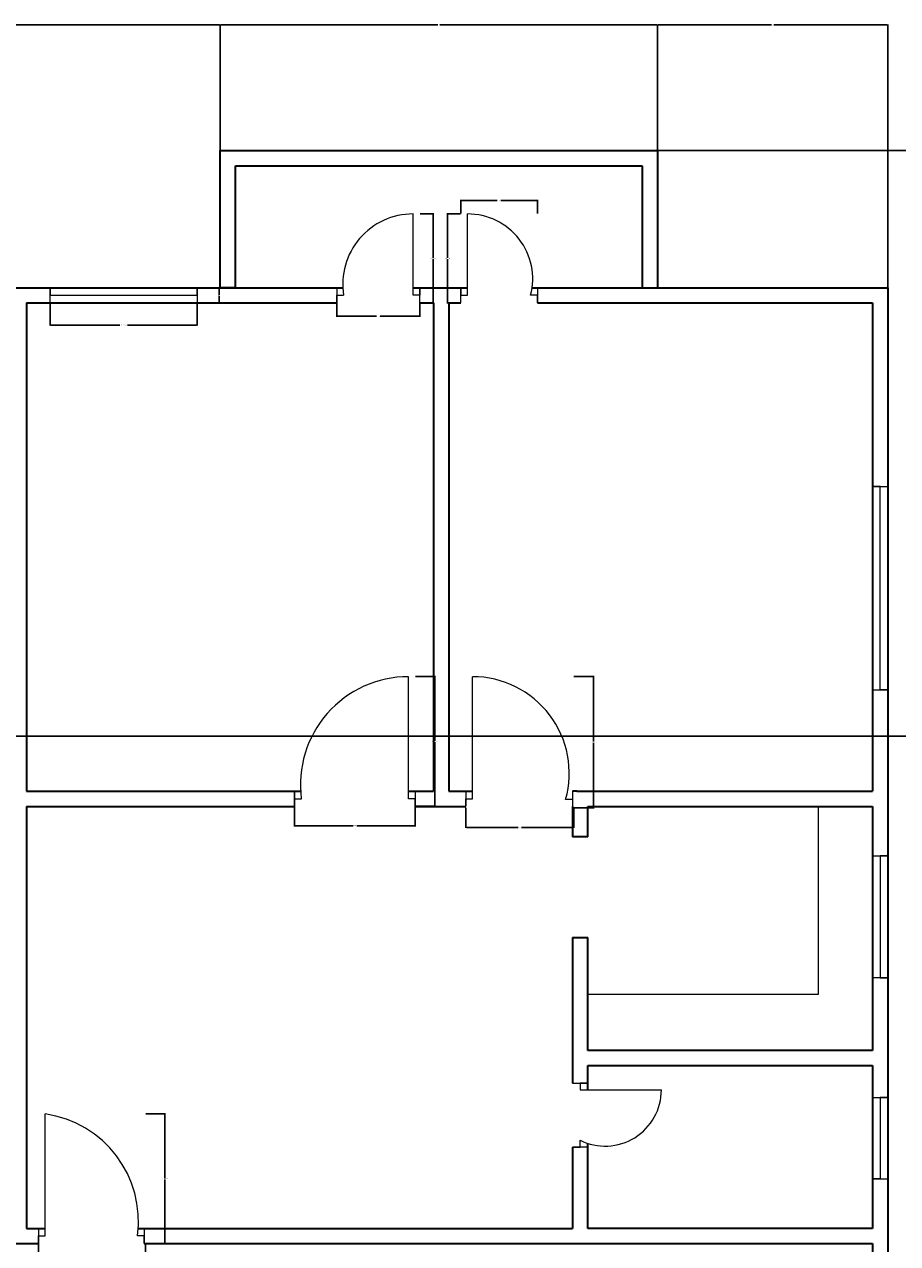
# Model space of a CAD drawing. Units: inches. Extents: x 1944 to 3454, y 1352 to 3055.
# Tile 14 of 17: x 2903 to 3160, y 1900 to 2260. Entities that reach past the tile are written whole.
import ezdxf

# ---------------------------------------------------------------- set-up
doc = ezdxf.new("R2010")
doc.units = ezdxf.units.IN
for name, color, linetype, lineweight in [('A-ANNO-DIMS', 2, 'Continuous', 18), ('A-ANNO-SYMB', 7, 'Continuous', 25), ('A-DOOR', 3, 'Continuous', 20), ('A-FLOR-CASE', 8, 'Continuous', 20), ('A-GLAZ', 4, 'Continuous', 18), ('A-WALL', 7, 'Continuous', 35)]:
    doc.layers.add(name, color=color, linetype=linetype, lineweight=lineweight)
doc.styles.get("Standard").update_dxf_attribs({"font": 'arial.ttf'})
doc.dimstyles.get("Standard").update_dxf_attribs({"dimtxt": 0.18, "dimasz": 0.18, "dimexe": 0.18, "dimexo": 0.0625, "dimgap": 0.09, "dimtad": 0, "dimtih": 1, "dimtoh": 1, "dimdec": 4, "dimzin": 0, "dimdsep": 46, "dimtxsty": 'Standard', "dimcen": 0.09, "dimadec": 0, "dimazin": 0, "dimtfac": 1, "dimtdec": 4, "dimtofl": 0, "dimtmove": 0, "dimatfit": 3, "dimfxl": 1, "dimtolj": 1, "dimtzin": 0, "dimarcsym": 0})

# ---------------------------------------------------------------- blocks, each defined once
blk = doc.blocks.new('DOOR-SWING-36IN-01')
for p, q in [((33.61, 2.25), (33.61, 38.25)), ((0, 4.5), (0, 0)), ((0, 0), (0, 4.5)), ((0, 4.5), (0, 2.25)), ((35.61, 4.5), (35.61, 0)), ((0, 2.25), (2, 2.25)), ((35.61, 2.25), (33.61, 2.25)), ((35.61, 0), (35.61, 2.25))]:
    blk.add_line(p, q)
blk.add_arc((33.61, 6.37), 31.88, 90, 187.4328)
blk = doc.blocks.new('DOOR-SWING-36IN-02')
for p, q in [((2, 2.65), (2, 38.65)), ((0, 4.9), (0, 0.4)), ((31.45, 4.9), (31.45, 0)), ((0, 0.4), (0, 2.65)), ((0, 2.65), (2, 2.65)), ((31.45, 2.45), (29.45, 2.45))]:
    blk.add_line(p, q)
blk.add_arc((2, 10.14), 28.51, 344.3464, 90)
blk = doc.blocks.new('DOOR-SWING-24IN-03')
for p, q in [((22.49, 2.25), (22.49, 26.25)), ((0, 4.5), (0, 0)), ((24.49, 0), (24.49, 4.5)), ((24.49, 4.5), (24.49, 2.25)), ((0, 0), (0, 2.25)), ((0, 2.25), (2, 2.25)), ((24.49, 2.25), (22.49, 2.25))]:
    blk.add_line(p, q)
blk.add_arc((22.49, 5.5), 20.75, 90, 189.0124)
blk = doc.blocks.new('DOOR-SWING-24IN-04')
for p, q in [((2, 2.25), (2, 26.25)), ((0, 0), (0, 4.5)), ((0, 4.5), (0, 2.25)), ((22.61, 4.5), (22.61, 0)), ((0, 2.25), (2, 2.25)), ((22.61, 2.25), (20.61, 2.25)), ((22.61, 0), (22.61, 2.25))]:
    blk.add_line(p, q)
blk.add_arc((2.1, 7.11), 19.14, 345.2922, 90.304)
blk = doc.blocks.new('DOOR-SWING-24IN-05')
for p, q in [((0, 18.87), (4.5, 18.87)), ((4.5, 18.87), (2.25, 18.87)), ((2.25, 18.87), (2.25, 16.87)), ((2.25, 16.87), (26.25, 16.87)), ((4.5, 0), (0, 0)), ((0, 0), (2.25, 0)), ((2.25, 0), (2.25, 2))]:
    blk.add_line(p, q)
blk.add_arc((9.64, 16.87), 16.61, 243.5781, 0)
blk = doc.blocks.new('DOOR-SWING-36IN-09')
for p, q in [((2, 2.25), (2, 38.25)), ((0, 4.5), (0, 0)), ((31.24, 4.5), (31.24, 0)), ((0, 0), (0, 2.25)), ((0, 2.25), (2, 2.25)), ((31.24, 2.25), (29.24, 2.25)), ((31.24, 0), (31.24, 2.25))]:
    blk.add_line(p, q)
blk.add_arc((-2.49, 6.55), 32.02, 352.2825, 81.9468)
blk = doc.blocks.new('WINDOW-PLAN-60.00IN-02')
for p, q in [((2.25, 60), (0, 60)), ((0, 60), (4.5, 60)), ((2.25, 0), (2.25, 60)), ((0, 0), (4.5, 0)), ((4.5, 0), (2.25, 0))]:
    blk.add_line(p, q)
blk = doc.blocks.new('WINDOW-PLAN-24.00IN-01')
for p, q in [((2.25, 24), (0, 24)), ((0, 24), (4.5, 24)), ((2.25, 0), (2.25, 24)), ((0, 0), (4.5, 0)), ((4.5, 0), (2.25, 0))]:
    blk.add_line(p, q)
blk = doc.blocks.new('WINDOW-PLAN-36.00IN-02')
for p, q in [((0, 36), (4.5, 36)), ((4.5, 36), (2.25, 36)), ((2.25, 36), (2.25, 0)), ((4.5, 0), (0, 0)), ((2.25, 0), (4.5, 0))]:
    blk.add_line(p, q)
blk = doc.blocks.new('WINDOW-PLAN-43.38IN-01')
for p, q in [((0, 0), (0, 4.5)), ((0, 4.5), (0, 2.25)), ((43.38, 2.25), (43.38, 4.5)), ((43.38, 4.5), (43.38, 0)), ((0, 2.25), (43.38, 2.25))]:
    blk.add_line(p, q)
blk = doc.blocks.new('*D88')
at = {"layer": 'A-ANNO-DIMS', "color": 0, "lineweight": -2, "transparency": 16777216}
for p, q in [((2910.28, 2177.53), (2910.28, 2170.91)), ((2953.65, 2177.53), (2953.65, 2170.91)), ((2910.46, 2171.09), (2930.85, 2171.09)), ((2953.47, 2171.09), (2933.08, 2171.09))]:
    blk.add_line(p, q, dxfattribs=at)
at = {"layer": 'A-ANNO-DIMS', "color": 0, "transparency": 16777216}
for points in [[(2910.46, 2171.12), (2910.46, 2171.06), (2910.28, 2171.09)], [(2953.47, 2171.12), (2953.47, 2171.06), (2953.65, 2171.09)]]:
    blk.add_solid(points, dxfattribs=at)
at = {"layer": 'Defpoints', "color": 0, "transparency": 16777216}
for p in [(2910.28, 2177.6), (2953.65, 2177.6), (2953.65, 2171.09)]:
    blk.add_point(p, dxfattribs=at)
at = {"layer": 'A-ANNO-DIMS', "color": 0, "transparency": 16777216, "insert": (2931.96, 2171.09), "char_height": 0.18, "attachment_point": 5}
blk.add_mtext('\\A1;WINDOW 43 TYP.', dxfattribs=at)
blk = doc.blocks.new('*D89')
at = {"layer": 'A-ANNO-DIMS', "color": 0, "lineweight": -2, "transparency": 16777216}
for p, q in [((2953.72, 2182.1), (2960.34, 2182.1)), ((2960.16, 2181.92), (2960.16, 2180.03)), ((2960.16, 2177.78), (2960.16, 2179.66)), ((2953.72, 2177.6), (2960.34, 2177.6))]:
    blk.add_line(p, q, dxfattribs=at)
at = {"layer": 'A-ANNO-DIMS', "color": 0, "transparency": 16777216}
for points in [[(2960.13, 2181.92), (2960.19, 2181.92), (2960.16, 2182.1)], [(2960.13, 2177.78), (2960.19, 2177.78), (2960.16, 2177.6)]]:
    blk.add_solid(points, dxfattribs=at)
at = {"layer": 'Defpoints', "color": 0, "transparency": 16777216}
for p in [(2953.65, 2182.1), (2960.16, 2182.1), (2953.65, 2177.6)]:
    blk.add_point(p, dxfattribs=at)
at = {"layer": 'A-ANNO-DIMS', "color": 0, "transparency": 16777216, "insert": (2960.16, 2179.85), "char_height": 0.18, "attachment_point": 5}
blk.add_mtext('\\A1;5 TYP.', dxfattribs=at)
blk = doc.blocks.new('*D92')
at = {"layer": 'A-ANNO-DIMS', "color": 0, "lineweight": -2, "transparency": 16777216}
for p, q in [((3018.08, 2067.35), (3023.94, 2067.35)), ((3023.76, 2067.17), (3023.76, 2048.4)), ((3023.76, 2029.28), (3023.76, 2048.04)), ((3018.08, 2029.1), (3023.94, 2029.1))]:
    blk.add_line(p, q, dxfattribs=at)
at = {"layer": 'A-ANNO-DIMS', "color": 0, "transparency": 16777216}
for points in [[(3023.73, 2067.17), (3023.79, 2067.17), (3023.76, 2067.35)], [(3023.73, 2029.28), (3023.79, 2029.28), (3023.76, 2029.1)]]:
    blk.add_solid(points, dxfattribs=at)
at = {"layer": 'Defpoints', "color": 0, "transparency": 16777216}
for p in [(3018.02, 2067.35), (3023.76, 2067.35), (3018.02, 2029.1)]:
    blk.add_point(p, dxfattribs=at)
at = {"layer": 'A-ANNO-DIMS', "color": 0, "transparency": 16777216, "insert": (3023.76, 2048.22), "char_height": 0.18, "attachment_point": 5}
blk.add_mtext('\\A1;SWING 38 TYP.', dxfattribs=at)
blk = doc.blocks.new('*D93')
at = {"layer": 'A-ANNO-DIMS', "color": 0, "lineweight": -2, "transparency": 16777216}
for p, q in [((2982.41, 2029.03), (2982.41, 2023.18)), ((3018.02, 2029.03), (3018.02, 2023.18)), ((2982.59, 2023.36), (2999.69, 2023.36)), ((3017.84, 2023.36), (3000.74, 2023.36))]:
    blk.add_line(p, q, dxfattribs=at)
at = {"layer": 'A-ANNO-DIMS', "color": 0, "transparency": 16777216}
for points in [[(2982.59, 2023.39), (2982.59, 2023.33), (2982.41, 2023.36)], [(3017.84, 2023.39), (3017.84, 2023.33), (3018.02, 2023.36)]]:
    blk.add_solid(points, dxfattribs=at)
at = {"layer": 'Defpoints', "color": 0, "transparency": 16777216}
for p in [(2982.41, 2029.1), (3018.02, 2029.1), (3018.02, 2023.36)]:
    blk.add_point(p, dxfattribs=at)
at = {"layer": 'A-ANNO-DIMS', "color": 0, "transparency": 16777216, "insert": (3000.21, 2023.36), "char_height": 0.18, "attachment_point": 5}
blk.add_mtext('\\A1;36 TYP.', dxfattribs=at)
blk = doc.blocks.new('*D94')
at = {"layer": 'A-ANNO-DIMS', "color": 0, "lineweight": -2, "transparency": 16777216}
for p, q in [((3064.84, 2067.35), (3070.76, 2067.35)), ((3070.58, 2067.17), (3070.58, 2048.21)), ((3070.58, 2028.88), (3070.58, 2047.84)), ((3064.84, 2028.7), (3070.76, 2028.7))]:
    blk.add_line(p, q, dxfattribs=at)
at = {"layer": 'A-ANNO-DIMS', "color": 0, "transparency": 16777216}
for points in [[(3070.55, 2067.17), (3070.61, 2067.17), (3070.58, 2067.35)], [(3070.55, 2028.88), (3070.61, 2028.88), (3070.58, 2028.7)]]:
    blk.add_solid(points, dxfattribs=at)
at = {"layer": 'Defpoints', "color": 0, "transparency": 16777216}
for p in [(3064.78, 2067.35), (3070.58, 2067.35), (3064.78, 2028.7)]:
    blk.add_point(p, dxfattribs=at)
at = {"layer": 'A-ANNO-DIMS', "color": 0, "transparency": 16777216, "insert": (3070.58, 2048.02), "char_height": 0.18, "attachment_point": 5}
blk.add_mtext('\\A1;SWING 39 TYP.', dxfattribs=at)
blk = doc.blocks.new('*D95')
at = {"layer": 'A-ANNO-DIMS', "color": 0, "lineweight": -2, "transparency": 16777216}
for p, q in [((3032.93, 2028.64), (3032.93, 2022.72)), ((3064.78, 2028.64), (3064.78, 2022.72)), ((3033.11, 2022.9), (3048.33, 2022.9)), ((3064.6, 2022.9), (3049.38, 2022.9))]:
    blk.add_line(p, q, dxfattribs=at)
at = {"layer": 'A-ANNO-DIMS', "color": 0, "transparency": 16777216}
for points in [[(3033.11, 2022.93), (3033.11, 2022.87), (3032.93, 2022.9)], [(3064.6, 2022.93), (3064.6, 2022.87), (3064.78, 2022.9)]]:
    blk.add_solid(points, dxfattribs=at)
at = {"layer": 'Defpoints', "color": 0, "transparency": 16777216}
for p in [(3032.93, 2028.7), (3064.78, 2028.7), (3064.78, 2022.9)]:
    blk.add_point(p, dxfattribs=at)
at = {"layer": 'A-ANNO-DIMS', "color": 0, "transparency": 16777216, "insert": (3048.85, 2022.9), "char_height": 0.18, "attachment_point": 5}
blk.add_mtext('\\A1;32 TYP.', dxfattribs=at)
blk = doc.blocks.new('*D108')
at = {"layer": 'A-ANNO-DIMS', "color": 0, "lineweight": -2, "transparency": 16777216}
for p, q in [((2938.5, 1938.35), (2944.35, 1938.35)), ((2944.17, 1938.17), (2944.17, 1919.4)), ((2944.17, 1900.28), (2944.17, 1919.04)), ((2938.5, 1900.1), (2944.35, 1900.1))]:
    blk.add_line(p, q, dxfattribs=at)
at = {"layer": 'A-ANNO-DIMS', "color": 0, "transparency": 16777216}
for points in [[(2944.14, 1938.17), (2944.2, 1938.17), (2944.17, 1938.35)], [(2944.14, 1900.28), (2944.2, 1900.28), (2944.17, 1900.1)]]:
    blk.add_solid(points, dxfattribs=at)
at = {"layer": 'Defpoints', "color": 0, "transparency": 16777216}
for p in [(2938.44, 1938.35), (2944.17, 1938.35), (2938.44, 1900.1)]:
    blk.add_point(p, dxfattribs=at)
at = {"layer": 'A-ANNO-DIMS', "color": 0, "transparency": 16777216, "insert": (2944.17, 1919.22), "char_height": 0.18, "attachment_point": 5}
blk.add_mtext('\\A1;SWING 38 TYP.', dxfattribs=at)
blk = doc.blocks.new('*D109')
at = {"layer": 'A-ANNO-DIMS', "color": 0, "lineweight": -2, "transparency": 16777216}
for p, q in [((2906.83, 1900.03), (2906.83, 1894.18)), ((2938.44, 1900.03), (2938.44, 1894.18)), ((2907.01, 1894.36), (2922.11, 1894.36)), ((2938.26, 1894.36), (2923.16, 1894.36))]:
    blk.add_line(p, q, dxfattribs=at)
at = {"layer": 'A-ANNO-DIMS', "color": 0, "transparency": 16777216}
for points in [[(2907.01, 1894.39), (2907.01, 1894.33), (2906.83, 1894.36)], [(2938.26, 1894.39), (2938.26, 1894.33), (2938.44, 1894.36)]]:
    blk.add_solid(points, dxfattribs=at)
at = {"layer": 'Defpoints', "color": 0, "transparency": 16777216}
for p in [(2906.83, 1900.1), (2938.44, 1900.1), (2938.44, 1894.36)]:
    blk.add_point(p, dxfattribs=at)
at = {"layer": 'A-ANNO-DIMS', "color": 0, "transparency": 16777216, "insert": (2922.63, 1894.36), "char_height": 0.18, "attachment_point": 5}
blk.add_mtext('\\A1;32 TYP.', dxfattribs=at)
blk = doc.blocks.new('*D120')
at = {"layer": 'A-ANNO-DIMS', "color": 0, "lineweight": -2, "transparency": 16777216}
for p, q in [((3019.44, 2203.85), (3023.5, 2203.85)), ((3023.32, 2203.67), (3023.32, 2190.9)), ((3023.32, 2177.78), (3023.32, 2190.54)), ((3019.44, 2177.6), (3023.5, 2177.6))]:
    blk.add_line(p, q, dxfattribs=at)
at = {"layer": 'A-ANNO-DIMS', "color": 0, "transparency": 16777216}
for points in [[(3023.29, 2203.67), (3023.35, 2203.67), (3023.32, 2203.85)], [(3023.29, 2177.78), (3023.35, 2177.78), (3023.32, 2177.6)]]:
    blk.add_solid(points, dxfattribs=at)
at = {"layer": 'Defpoints', "color": 0, "transparency": 16777216}
for p in [(3019.38, 2203.85), (3023.32, 2203.85), (3019.38, 2177.6)]:
    blk.add_point(p, dxfattribs=at)
at = {"layer": 'A-ANNO-DIMS', "color": 0, "transparency": 16777216, "insert": (3023.32, 2190.72), "char_height": 0.18, "attachment_point": 5}
blk.add_mtext('\\A1;SWING 26 TYP.', dxfattribs=at)
blk = doc.blocks.new('*D121')
at = {"layer": 'A-ANNO-DIMS', "color": 0, "lineweight": -2, "transparency": 16777216}
for p, q in [((2994.89, 2177.53), (2994.89, 2173.48)), ((3019.38, 2177.53), (3019.38, 2173.48)), ((2995.07, 2173.66), (3006.6, 2173.66)), ((3019.2, 2173.66), (3007.66, 2173.66))]:
    blk.add_line(p, q, dxfattribs=at)
at = {"layer": 'A-ANNO-DIMS', "color": 0, "transparency": 16777216}
for points in [[(2995.07, 2173.69), (2995.07, 2173.63), (2994.89, 2173.66)], [(3019.2, 2173.69), (3019.2, 2173.63), (3019.38, 2173.66)]]:
    blk.add_solid(points, dxfattribs=at)
at = {"layer": 'Defpoints', "color": 0, "transparency": 16777216}
for p in [(2994.89, 2177.6), (3019.38, 2177.6), (3019.38, 2173.66)]:
    blk.add_point(p, dxfattribs=at)
at = {"layer": 'A-ANNO-DIMS', "color": 0, "transparency": 16777216, "insert": (3007.13, 2173.66), "char_height": 0.18, "attachment_point": 5}
blk.add_mtext('\\A1;24 TYP.', dxfattribs=at)
blk = doc.blocks.new('*D122')
at = {"layer": 'A-ANNO-DIMS', "color": 0, "lineweight": -2, "transparency": 16777216}
for p, q in [((3031.36, 2203.88), (3027.3, 2203.88)), ((3027.48, 2203.7), (3027.48, 2190.92)), ((3027.48, 2177.78), (3027.48, 2190.55)), ((3031.36, 2177.6), (3027.3, 2177.6))]:
    blk.add_line(p, q, dxfattribs=at)
at = {"layer": 'A-ANNO-DIMS', "color": 0, "transparency": 16777216}
for points in [[(3027.45, 2203.7), (3027.51, 2203.7), (3027.48, 2203.88)], [(3027.45, 2177.78), (3027.51, 2177.78), (3027.48, 2177.6)]]:
    blk.add_solid(points, dxfattribs=at)
at = {"layer": 'Defpoints', "color": 0, "transparency": 16777216}
for p in [(3027.48, 2203.88), (3031.42, 2203.88), (3031.42, 2177.6)]:
    blk.add_point(p, dxfattribs=at)
at = {"layer": 'A-ANNO-DIMS', "color": 0, "transparency": 16777216, "insert": (3027.48, 2190.74), "char_height": 0.18, "attachment_point": 5}
blk.add_mtext('\\A1;SWING 26 TYP.', dxfattribs=at)
blk = doc.blocks.new('*D123')
at = {"layer": 'A-ANNO-DIMS', "color": 0, "lineweight": -2, "transparency": 16777216}
for p, q in [((3031.42, 2203.94), (3031.42, 2208)), ((3031.6, 2207.82), (3042.2, 2207.82)), ((3053.85, 2207.82), (3043.26, 2207.82)), ((3054.03, 2203.94), (3054.03, 2208))]:
    blk.add_line(p, q, dxfattribs=at)
at = {"layer": 'A-ANNO-DIMS', "color": 0, "transparency": 16777216}
for points in [[(3031.6, 2207.85), (3031.6, 2207.79), (3031.42, 2207.82)], [(3053.85, 2207.85), (3053.85, 2207.79), (3054.03, 2207.82)]]:
    blk.add_solid(points, dxfattribs=at)
at = {"layer": 'Defpoints', "color": 0, "transparency": 16777216}
for p in [(3054.03, 2207.82), (3031.42, 2203.88), (3054.03, 2203.88)]:
    blk.add_point(p, dxfattribs=at)
at = {"layer": 'A-ANNO-DIMS', "color": 0, "transparency": 16777216, "insert": (3042.73, 2207.82), "char_height": 0.18, "attachment_point": 5}
blk.add_mtext('\\A1;23 TYP.', dxfattribs=at)
blk = doc.blocks.new('*D187')
at = {"layer": 'A-ANNO-DIMS', "color": 0, "lineweight": -2, "transparency": 16777216}
for p, q in [((3089.53, 2222.6), (3245.46, 2222.6)), ((3245.28, 2222.42), (3245.28, 1856.28)), ((3245.28, 1489.78), (3245.28, 1855.91)), ((3093.18, 1489.6), (3245.46, 1489.6))]:
    blk.add_line(p, q, dxfattribs=at)
at = {"layer": 'A-ANNO-DIMS', "color": 0, "transparency": 16777216}
for points in [[(3245.25, 2222.42), (3245.31, 2222.42), (3245.28, 2222.6)], [(3245.25, 1489.78), (3245.31, 1489.78), (3245.28, 1489.6)]]:
    blk.add_solid(points, dxfattribs=at)
at = {"layer": 'Defpoints', "color": 0, "transparency": 16777216}
for p in [(3089.47, 2222.6), (3245.28, 2222.6), (3093.12, 1489.6)]:
    blk.add_point(p, dxfattribs=at)
at = {"layer": 'A-ANNO-DIMS', "color": 0, "transparency": 16777216, "insert": (3245.28, 1856.1), "char_height": 0.18, "attachment_point": 5}
blk.add_mtext('\\A1;733', dxfattribs=at)
blk = doc.blocks.new('*D196')
at = {"layer": 'A-ANNO-DIMS', "color": 0, "lineweight": -2, "transparency": 16777216}
for p, q in [((2838.72, 2222.66), (2838.72, 2259.78)), ((2838.9, 2259.6), (2899.14, 2259.6)), ((2960.29, 2259.6), (2900.05, 2259.6)), ((2960.47, 2222.66), (2960.47, 2259.78))]:
    blk.add_line(p, q, dxfattribs=at)
at = {"layer": 'A-ANNO-DIMS', "color": 0, "transparency": 16777216}
for points in [[(2838.9, 2259.63), (2838.9, 2259.57), (2838.72, 2259.6)], [(2960.29, 2259.63), (2960.29, 2259.57), (2960.47, 2259.6)]]:
    blk.add_solid(points, dxfattribs=at)
at = {"layer": 'Defpoints', "color": 0, "transparency": 16777216}
for p in [(2960.47, 2259.6), (2838.72, 2222.6), (2960.47, 2222.6)]:
    blk.add_point(p, dxfattribs=at)
at = {"layer": 'A-ANNO-DIMS', "color": 0, "transparency": 16777216, "insert": (2899.6, 2259.6), "char_height": 0.18, "attachment_point": 5}
blk.add_mtext('\\A1;121.75', dxfattribs=at)
blk = doc.blocks.new('*D197')
at = {"layer": 'A-ANNO-DIMS', "color": 0, "lineweight": -2, "transparency": 16777216}
for p, q in [((2960.47, 2222.66), (2960.47, 2259.78)), ((2960.65, 2259.6), (3024.69, 2259.6)), ((3089.29, 2259.6), (3025.25, 2259.6)), ((3089.47, 2222.66), (3089.47, 2259.78))]:
    blk.add_line(p, q, dxfattribs=at)
at = {"layer": 'A-ANNO-DIMS', "color": 0, "transparency": 16777216}
for points in [[(2960.65, 2259.63), (2960.65, 2259.57), (2960.47, 2259.6)], [(3089.29, 2259.63), (3089.29, 2259.57), (3089.47, 2259.6)]]:
    blk.add_solid(points, dxfattribs=at)
at = {"layer": 'Defpoints', "color": 0, "transparency": 16777216}
for p in [(3089.47, 2259.6), (2960.47, 2222.6), (3089.47, 2222.6)]:
    blk.add_point(p, dxfattribs=at)
at = {"layer": 'A-ANNO-DIMS', "color": 0, "transparency": 16777216, "insert": (3024.97, 2259.6), "char_height": 0.18, "attachment_point": 5}
blk.add_mtext('\\A1;129', dxfattribs=at)
blk = doc.blocks.new('*D198')
at = {"layer": 'A-ANNO-DIMS', "color": 0, "lineweight": -2, "transparency": 16777216}
for p, q in [((3089.47, 2222.66), (3089.47, 2259.78)), ((3089.65, 2259.6), (3123.1, 2259.6)), ((3157.2, 2259.6), (3123.75, 2259.6)), ((3157.38, 2182.16), (3157.38, 2259.78))]:
    blk.add_line(p, q, dxfattribs=at)
at = {"layer": 'A-ANNO-DIMS', "color": 0, "transparency": 16777216}
for points in [[(3089.65, 2259.63), (3089.65, 2259.57), (3089.47, 2259.6)], [(3157.2, 2259.63), (3157.2, 2259.57), (3157.38, 2259.6)]]:
    blk.add_solid(points, dxfattribs=at)
at = {"layer": 'Defpoints', "color": 0, "transparency": 16777216}
for p in [(3157.38, 2259.6), (3089.47, 2222.6), (3157.38, 2182.1)]:
    blk.add_point(p, dxfattribs=at)
at = {"layer": 'A-ANNO-DIMS', "color": 0, "transparency": 16777216, "insert": (3123.42, 2259.6), "char_height": 0.18, "attachment_point": 5}
blk.add_mtext('\\A1;67.9', dxfattribs=at)

msp = doc.modelspace()

# ---------------------------------------------------------------- linework, layer by layer
at = {"layer": 'A-ANNO-SYMB'}
msp.add_line((2622.416, 2049.778), (3208.282, 2049.778), dxfattribs=at)
at = {"layer": 'A-FLOR-CASE'}
for p, q in [((3137.007, 1973.733), (3137.007, 2029.096)), ((3068.875, 1973.733), (3137.007, 1973.733))]:
    msp.add_line(p, q, dxfattribs=at)
at = {"layer": 'A-WALL'}
for p, q in [((2960.47, 2218.096), (2960.47, 2222.596)), ((2960.47, 2222.596), (3084.97, 2222.596)), ((3084.97, 2222.596), (3089.47, 2222.596)), ((3089.47, 2222.596), (3089.47, 2182.096)), ((2960.47, 2182.096), (2960.47, 2218.096)), ((2964.97, 2182.096), (2964.97, 2218.096)), ((2964.97, 2218.096), (3084.97, 2218.096)), ((3084.97, 2218.096), (3084.97, 2182.096)), ((2804.773, 2182.096), (2996.655, 2182.096)), ((2964.97, 2182.096), (2960.47, 2182.096)), ((3017.381, 2182.096), (3033.419, 2182.096)), ((3052.483, 2182.096), (3157.375, 2182.096)), ((3157.375, 2182.096), (3157.375, 1530.096)), ((2903.375, 2177.596), (2994.887, 2177.596)), ((2903.375, 2177.596), (2903.375, 2033.596)), ((3019.381, 2177.596), (3023.375, 2177.596)), ((3023.375, 2177.596), (3023.375, 2033.596)), ((3027.875, 2177.596), (3031.419, 2177.596)), ((3027.875, 2177.596), (3027.875, 2033.596)), ((3054.034, 2177.596), (3152.875, 2177.596)), ((3152.875, 2177.596), (3152.875, 2033.596)), ((2903.375, 2033.596), (2984.196, 2033.596)), ((3016.018, 2033.596), (3023.375, 2033.596)), ((3027.875, 2033.596), (3034.926, 2033.596)), ((3065.634, 2033.596), (3064.375, 2033.596)), ((3065.634, 2033.596), (3152.875, 2033.596)), ((2903.375, 2029.096), (2982.409, 2029.096)), ((2903.375, 2029.096), (2903.375, 1904.596)), ((3018.018, 2029.096), (3032.926, 2029.096)), ((3064.375, 2029.096), (3064.375, 2020.069)), ((3068.875, 2029.096), (3152.875, 2029.096)), ((3068.875, 2020.069), (3068.875, 2029.096)), ((3152.875, 2029.096), (3152.875, 1957.096)), ((3152.875, 2029.096), (3152.875, 1957.096)), ((3068.875, 2020.069), (3064.375, 2020.069)), ((3064.375, 1990.369), (3064.375, 1957.096)), ((3064.375, 1990.369), (3068.875, 1990.369)), ((3068.875, 1957.096), (3068.875, 1990.369)), ((3064.375, 1957.096), (3064.375, 1952.596)), ((3152.875, 1957.096), (3068.875, 1957.096)), ((3064.375, 1952.596), (3064.375, 1947.471)), ((3068.875, 1952.596), (3152.875, 1952.596)), ((3068.875, 1945.471), (3068.875, 1952.596)), ((3152.875, 1952.596), (3152.875, 1904.596)), ((3152.875, 1952.596), (3152.875, 1904.596)), ((3064.375, 1928.596), (3064.375, 1904.596)), ((3068.875, 1904.596), (3068.875, 1929.677)), ((2903.375, 1904.596), (2908.831, 1904.596)), ((2936.296, 1904.596), (3064.375, 1904.596)), ((3152.875, 1904.596), (3068.875, 1904.596)), ((2895.494, 1900.096), (2906.831, 1900.096)), ((2938.072, 1900.096), (3064.375, 1900.096)), ((3064.375, 1900.096), (3152.875, 1900.096)), ((3152.875, 1900.096), (3152.875, 1840.096)), ((3152.875, 1900.096), (3152.875, 1895.596))]:
    msp.add_line(p, q, dxfattribs=at)

# ---------------------------------------------------------------- block references
at = {"layer": 'A-DOOR'}
for name, p in [('DOOR-SWING-24IN-03', (2994.888, 2177.596)), ('DOOR-SWING-24IN-04', (3031.42, 2177.596)), ('DOOR-SWING-36IN-01', (2982.409, 2029.096)), ('DOOR-SWING-36IN-02', (3032.926, 2028.698)), ('DOOR-SWING-24IN-05', (3064.376, 1928.596)), ('DOOR-SWING-36IN-09', (2906.831, 1900.096))]:
    msp.add_blockref(name, p, dxfattribs=at)
at = {"layer": 'A-GLAZ'}
for name, p in [('WINDOW-PLAN-43.38IN-01', (2910.276, 2177.596)), ('WINDOW-PLAN-60.00IN-02', (3152.876, 2063.452)), ('WINDOW-PLAN-36.00IN-02', (3152.876, 1978.5))]:
    msp.add_blockref(name, p, dxfattribs=at)
at = {"layer": 'A-GLAZ', "extrusion": (0, 0, -1), "zscale": -1, "rotation": 180}
msp.add_blockref('WINDOW-PLAN-24.00IN-01', (-3152.876, 1943.2), dxfattribs=at)

# ---------------------------------------------------------------- dimensions: what is measured, and where the dimension line sits
at = {"layer": 'A-ANNO-DIMS'}
for base, p1, p2, override, picture, middle in [((2960.47, 2259.596), (2838.721, 2222.596), (2960.47, 2222.596), {"dimdec": 2, "dimlfac": 1, "dimrnd": 0, "dimzin": 0, "dimdsep": 46, "dimlunit": 2}, '*D196', (2899.596, 2259.596)), ((3089.47, 2259.596), (2960.47, 2222.596), (3089.47, 2222.596), {"dimdec": 0, "dimlfac": 1, "dimrnd": 0, "dimzin": 0, "dimdsep": 46, "dimlunit": 2}, '*D197', (3024.97, 2259.596)), ((3157.375, 2259.596), (3089.47, 2222.596), (3157.375, 2182.096), {"dimdec": 1, "dimlfac": 1, "dimrnd": 0, "dimzin": 0, "dimdsep": 46, "dimlunit": 2}, '*D198', (3123.423, 2259.596))]:
    dim = msp.add_linear_dim(base=base, p1=p1, p2=p2, dimstyle='Standard', override=override, dxfattribs=at)
    dim.commit()
    dim.dimension.update_dxf_attribs({"geometry": picture, "text_midpoint": middle})
dim = msp.add_linear_dim(base=(3245.282, 2222.596), p1=(3093.12, 1489.596), p2=(3089.47, 2222.596), angle=90, dimstyle='Standard', override={"dimdec": 0, "dimlfac": 1, "dimrnd": 0, "dimzin": 0, "dimdsep": 46, "dimlunit": 2}, dxfattribs=at)
dim.commit()
dim.dimension.update_dxf_attribs({"geometry": '*D187', "text_midpoint": (3245.282, 1856.096)})
for base, p1, p2, text, picture, middle in [((3054.034, 2207.82), (3031.419, 2203.878), (3054.034, 2203.878), '<> TYP.', '*D123', (3042.727, 2207.82)), ((2953.653, 2171.09), (2910.276, 2177.596), (2953.653, 2177.596), 'WINDOW <> TYP.', '*D88', (2931.964, 2171.09)), ((3019.381, 2173.659), (2994.887, 2177.596), (3019.381, 2177.596), '<> TYP.', '*D121', (3007.134, 2173.659)), ((3018.018, 2023.359), (2982.409, 2029.096), (3018.018, 2029.096), '<> TYP.', '*D93', (3000.213, 2023.359)), ((3064.782, 2022.901), (3032.926, 2028.698), (3064.782, 2028.698), '<> TYP.', '*D95', (3048.854, 2022.901)), ((2938.437, 1894.359), (2906.831, 1900.096), (2938.437, 1900.096), '<> TYP.', '*D109', (2922.634, 1894.359))]:
    dim = msp.add_linear_dim(base=base, p1=p1, p2=p2, text=text, dimstyle='Standard', override={"dimdec": 0, "dimlfac": 1, "dimrnd": 0, "dimzin": 0, "dimdsep": 46, "dimlunit": 2}, dxfattribs=at)
    dim.commit()
    dim.dimension.update_dxf_attribs({"geometry": picture, "text_midpoint": middle})
for base, p1, p2, text, picture, middle in [((3023.318, 2203.846), (3019.381, 2177.596), (3019.381, 2203.846), 'SWING <> TYP.', '*D120', (3023.318, 2190.721)), ((3027.477, 2203.878), (3031.419, 2177.596), (3031.419, 2203.878), 'SWING <> TYP.', '*D122', (3027.477, 2190.737)), ((2960.159904358, 2182.096365033), (2953.653260314, 2177.596365033), (2953.653260314, 2182.096365033), '<> TYP.', '*D89', (2960.159904358, 2179.846365033)), ((3023.755, 2067.346), (3018.018, 2029.096), (3018.018, 2067.346), 'SWING <> TYP.', '*D92', (3023.755, 2048.221)), ((3070.579, 2067.346), (3064.782, 2028.698), (3064.782, 2067.346), 'SWING <> TYP.', '*D94', (3070.579, 2048.022)), ((2944.174, 1938.346), (2938.437, 1900.096), (2938.437, 1938.346), 'SWING <> TYP.', '*D108', (2944.174, 1919.221))]:
    dim = msp.add_linear_dim(base=base, p1=p1, p2=p2, angle=90, text=text, dimstyle='Standard', override={"dimdec": 0, "dimlfac": 1, "dimrnd": 0, "dimzin": 0, "dimdsep": 46, "dimlunit": 2}, dxfattribs=at)
    dim.commit()
    dim.dimension.update_dxf_attribs({"geometry": picture, "text_midpoint": middle})

doc.saveas('drawing.dxf')
